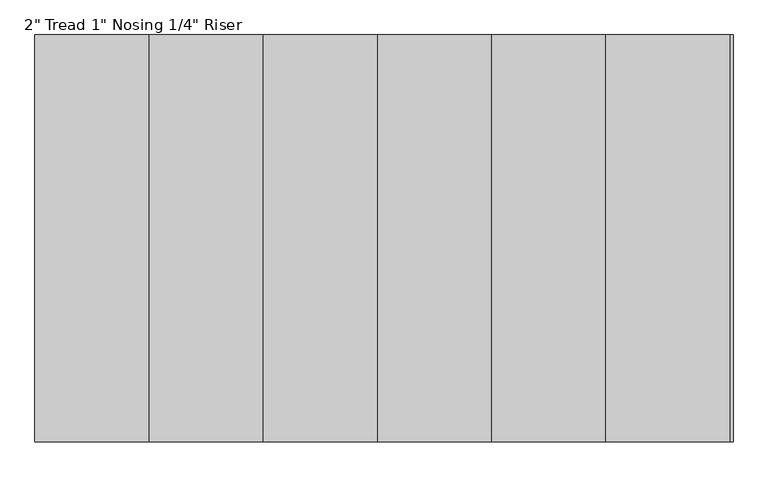
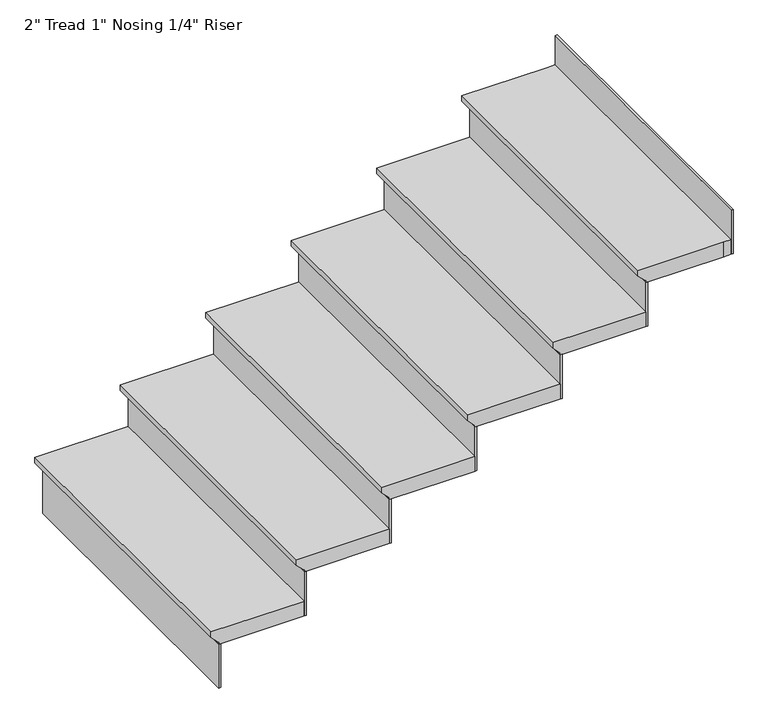
"""IFC4 building model written with IfcOpenShell, lengths in millimetres: stair flight geometry."""

from ifc_helpers import new_model, si_unit, origin, place, context, project, spatial, faceted_brep, source, transform, mapped, element, save


def stair_flight_69e76367(model_context):
    return source(origin(), model_context, "Body", "Brep", [
        faceted_brep([(-6729.7502524, 11195.5128362, 4857.75), (-6729.7502524, 11195.5128362, 4876.8), (-6729.7502524, 12192.4628362, 4876.8), (-6729.7502524, 12192.4628362, 4857.75), (-6704.3502524, 11195.5128362, 4832.35), (-6704.3502524, 12192.4628362, 4832.35), (-6424.9502524, 11195.5128362, 4876.8), (-6424.9502524, 12192.4628362, 4876.8), (-6704.3502524, 12192.4628362, 4826.0), (-6424.9502524, 12192.4628362, 4826.0), (-6424.9502524, 11195.5128362, 4826.0), (-6704.3502524, 11195.5128362, 4826.0)], [[[0, 1, 2, 3]], [[4, 0, 3, 5]], [[2, 1, 6, 7]], [[8, 9, 10, 11]], [[2, 7, 9, 8, 5, 3]], [[8, 11, 4, 5]], [[6, 1, 0, 4, 11, 10]], [[7, 6, 10, 9]]]),
        faceted_brep([(-6704.3502524, 11195.5128362, 4826.0), (-6704.3502524, 11195.5128362, 4673.6), (-6698.0002524, 11195.5128362, 4673.6), (-6698.0002524, 11195.5128362, 4826.0), (-6704.3502524, 12192.4628362, 4826.0), (-6698.0002524, 12192.4628362, 4826.0), (-6698.0002524, 12192.4628362, 4673.6), (-6704.3502524, 12192.4628362, 4673.6)], [[[0, 1, 2, 3]], [[4, 5, 6, 7]], [[1, 0, 4, 7]], [[2, 1, 7, 6]], [[3, 2, 6, 5]], [[0, 3, 5, 4]]]),
        faceted_brep([(-6424.9502524, 11195.5128362, 4978.4), (-6424.9502524, 11195.5128362, 4826.0), (-6418.6002524, 11195.5128362, 4826.0), (-6418.6002524, 11195.5128362, 4978.4), (-6424.9502524, 12192.4628362, 4978.4), (-6418.6002524, 12192.4628362, 4978.4), (-6418.6002524, 12192.4628362, 4826.0), (-6424.9502524, 12192.4628362, 4826.0)], [[[0, 1, 2, 3]], [[4, 5, 6, 7]], [[1, 0, 4, 7]], [[2, 1, 7, 6]], [[3, 2, 6, 5]], [[0, 3, 5, 4]]]),
        faceted_brep([(-6450.3502524, 12192.4628362, 5029.2), (-6450.3502524, 11195.5128362, 5029.2), (-6145.5502524, 11195.5128362, 5029.2), (-6145.5502524, 12192.4628362, 5029.2), (-6424.9502524, 12192.4628362, 4978.4), (-6145.5502524, 12192.4628362, 4978.4), (-6145.5502524, 11195.5128362, 4978.4), (-6424.9502524, 11195.5128362, 4978.4), (-6424.9502524, 12192.4628362, 4984.75), (-6450.3502524, 12192.4628362, 5010.15), (-6424.9502524, 11195.5128362, 4984.75), (-6450.3502524, 11195.5128362, 5010.15)], [[[0, 1, 2, 3]], [[4, 5, 6, 7]], [[0, 3, 5, 4, 8, 9]], [[4, 7, 10, 8]], [[2, 1, 11, 10, 7, 6]], [[3, 2, 6, 5]], [[11, 1, 0, 9]], [[10, 11, 9, 8]]]),
        faceted_brep([(-6145.5502524, 11195.5128362, 5130.8), (-6145.5502524, 11195.5128362, 4978.4), (-6139.2002524, 11195.5128362, 4978.4), (-6139.2002524, 11195.5128362, 5130.8), (-6145.5502524, 12192.4628362, 5130.8), (-6139.2002524, 12192.4628362, 5130.8), (-6139.2002524, 12192.4628362, 4978.4), (-6145.5502524, 12192.4628362, 4978.4)], [[[0, 1, 2, 3]], [[4, 5, 6, 7]], [[1, 0, 4, 7]], [[2, 1, 7, 6]], [[3, 2, 6, 5]], [[0, 3, 5, 4]]]),
        faceted_brep([(-6170.9502524, 12192.4628362, 5181.6), (-6170.9502524, 11195.5128362, 5181.6), (-5866.1502524, 11195.5128362, 5181.6), (-5866.1502524, 12192.4628362, 5181.6), (-6145.5502524, 12192.4628362, 5130.8), (-5866.1502524, 12192.4628362, 5130.8), (-5866.1502524, 11195.5128362, 5130.8), (-6145.5502524, 11195.5128362, 5130.8), (-6145.5502524, 12192.4628362, 5137.15), (-6170.9502524, 12192.4628362, 5162.55), (-6145.5502524, 11195.5128362, 5137.15), (-6170.9502524, 11195.5128362, 5162.55)], [[[0, 1, 2, 3]], [[4, 5, 6, 7]], [[0, 3, 5, 4, 8, 9]], [[4, 7, 10, 8]], [[2, 1, 11, 10, 7, 6]], [[3, 2, 6, 5]], [[11, 1, 0, 9]], [[10, 11, 9, 8]]]),
        faceted_brep([(-5866.1502524, 11195.5128362, 5283.2), (-5866.1502524, 11195.5128362, 5130.8), (-5859.8002524, 11195.5128362, 5130.8), (-5859.8002524, 11195.5128362, 5283.2), (-5866.1502524, 12192.4628362, 5283.2), (-5859.8002524, 12192.4628362, 5283.2), (-5859.8002524, 12192.4628362, 5130.8), (-5866.1502524, 12192.4628362, 5130.8)], [[[0, 1, 2, 3]], [[4, 5, 6, 7]], [[1, 0, 4, 7]], [[2, 1, 7, 6]], [[3, 2, 6, 5]], [[0, 3, 5, 4]]]),
        faceted_brep([(-5891.5502524, 12192.4628362, 5334.0), (-5891.5502524, 11195.5128362, 5334.0), (-5586.7502524, 11195.5128362, 5334.0), (-5586.7502524, 12192.4628362, 5334.0), (-5866.1502524, 12192.4628362, 5283.2), (-5586.7502524, 12192.4628362, 5283.2), (-5586.7502524, 11195.5128362, 5283.2), (-5866.1502524, 11195.5128362, 5283.2), (-5866.1502524, 12192.4628362, 5289.55), (-5891.5502524, 12192.4628362, 5314.95), (-5866.1502524, 11195.5128362, 5289.55), (-5891.5502524, 11195.5128362, 5314.95)], [[[0, 1, 2, 3]], [[4, 5, 6, 7]], [[0, 3, 5, 4, 8, 9]], [[4, 7, 10, 8]], [[2, 1, 11, 10, 7, 6]], [[3, 2, 6, 5]], [[11, 1, 0, 9]], [[10, 11, 9, 8]]]),
        faceted_brep([(-5586.7502524, 11195.5128362, 5435.6), (-5586.7502524, 11195.5128362, 5283.2), (-5580.4002524, 11195.5128362, 5283.2), (-5580.4002524, 11195.5128362, 5435.6), (-5586.7502524, 12192.4628362, 5435.6), (-5580.4002524, 12192.4628362, 5435.6), (-5580.4002524, 12192.4628362, 5283.2), (-5586.7502524, 12192.4628362, 5283.2)], [[[0, 1, 2, 3]], [[4, 5, 6, 7]], [[1, 0, 4, 7]], [[2, 1, 7, 6]], [[3, 2, 6, 5]], [[0, 3, 5, 4]]]),
        faceted_brep([(-5612.1502524, 12192.4628362, 5486.4), (-5612.1502524, 11195.5128362, 5486.4), (-5307.3502524, 11195.5128362, 5486.4), (-5307.3502524, 12192.4628362, 5486.4), (-5586.7502524, 12192.4628362, 5435.6), (-5307.3502524, 12192.4628362, 5435.6), (-5307.3502524, 11195.5128362, 5435.6), (-5586.7502524, 11195.5128362, 5435.6), (-5586.7502524, 12192.4628362, 5441.95), (-5612.1502524, 12192.4628362, 5467.35), (-5586.7502524, 11195.5128362, 5441.95), (-5612.1502524, 11195.5128362, 5467.35)], [[[0, 1, 2, 3]], [[4, 5, 6, 7]], [[0, 3, 5, 4, 8, 9]], [[4, 7, 10, 8]], [[2, 1, 11, 10, 7, 6]], [[3, 2, 6, 5]], [[11, 1, 0, 9]], [[10, 11, 9, 8]]]),
        faceted_brep([(-5027.9502524, 11195.5128362, 5740.4), (-5027.9502524, 11195.5128362, 5588.0), (-5021.6002524, 11195.5128362, 5588.0), (-5021.6002524, 11195.5128362, 5740.4), (-5027.9502524, 12192.4628362, 5740.4), (-5021.6002524, 12192.4628362, 5740.4), (-5021.6002524, 12192.4628362, 5588.0), (-5027.9502524, 12192.4628362, 5588.0)], [[[0, 1, 2, 3]], [[4, 5, 6, 7]], [[1, 0, 4, 7]], [[2, 1, 7, 6]], [[3, 2, 6, 5]], [[0, 3, 5, 4]]]),
        faceted_brep([(-5307.3502524, 11195.5128362, 5588.0), (-5307.3502524, 11195.5128362, 5435.6), (-5301.0002524, 11195.5128362, 5435.6), (-5301.0002524, 11195.5128362, 5588.0), (-5307.3502524, 12192.4628362, 5588.0), (-5301.0002524, 12192.4628362, 5588.0), (-5301.0002524, 12192.4628362, 5435.6), (-5307.3502524, 12192.4628362, 5435.6)], [[[0, 1, 2, 3]], [[4, 5, 6, 7]], [[1, 0, 4, 7]], [[2, 1, 7, 6]], [[3, 2, 6, 5]], [[0, 3, 5, 4]]]),
        faceted_brep([(-5027.9502524, 12192.4628362, 5638.8), (-5053.3502524, 12192.4628362, 5638.8), (-5332.7502524, 12192.4628362, 5638.8), (-5332.7502524, 11195.5128362, 5638.8), (-5053.3502524, 11195.5128362, 5638.8), (-5027.9502524, 11195.5128362, 5638.8), (-5053.3502524, 12192.4628362, 5588.0), (-5027.9502524, 12192.4628362, 5588.0), (-5027.9502524, 11195.5128362, 5588.0), (-5053.3502524, 11195.5128362, 5588.0), (-5307.3502524, 11195.5128362, 5588.0), (-5307.3502524, 12192.4628362, 5588.0), (-5307.3502524, 12192.4628362, 5594.35), (-5332.7502524, 12192.4628362, 5619.75), (-5307.3502524, 11195.5128362, 5594.35), (-5332.7502524, 11195.5128362, 5619.75)], [[[0, 1, 2, 3, 4, 5]], [[6, 7, 8, 9, 10, 11]], [[1, 0, 7, 6]], [[2, 1, 6, 11, 12, 13]], [[11, 10, 14, 12]], [[4, 3, 15, 14, 10, 9]], [[5, 4, 9, 8]], [[0, 5, 8, 7]], [[15, 3, 2, 13]], [[14, 15, 13, 12]]]),
    ])


if __name__ == "__main__":
    model = new_model("IFC4")
    model_context = context("Model", 3, world=origin())
    ifc_project = project(units=[si_unit("LENGTHUNIT", "METRE", prefix="MILLI")], contexts=[model_context])
    site = spatial("IfcSite", under=ifc_project)
    building = spatial("IfcBuilding", under=site)
    placement = place(None, origin())
    stair_flight_shape = stair_flight_69e76367(model_context)
    element("IfcStairFlight", 1, ObjectType="2\" Tread 1\" Nosing 1/4\" Riser", at=placement, inside=building, context=model_context, shape_type="MappedRepresentation", body=[
        mapped(stair_flight_shape, transform((0.0, 0.0, 0.0), x_axis=(1.0, 0.0, 0.0), y_axis=(0.0, 1.0, 0.0), z_axis=(0.0, 0.0, 1.0))),
    ])
    save(model, "model.ifc")
